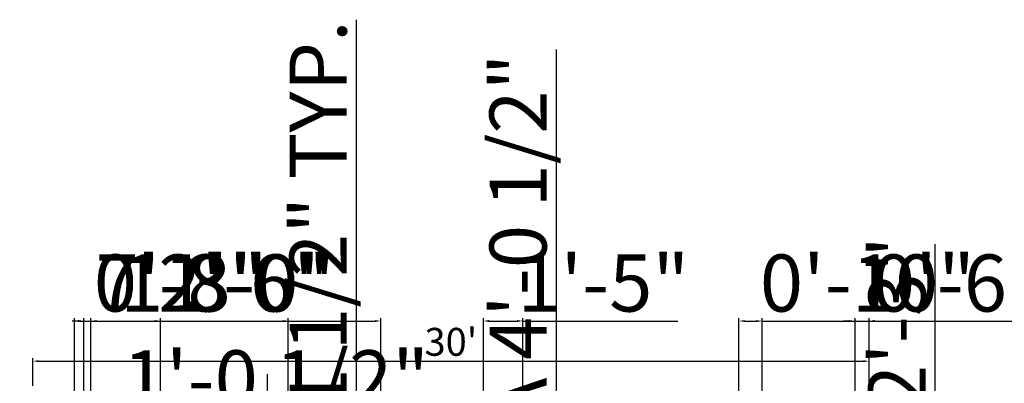
# Model space of a CAD drawing. Units: inches. Extents: x 1542 to 2523, y 1699 to 2449.
# Tile 6 of 7: x 1875 to 2299, y 2292 to 2449. Entities that reach past the tile are written whole.
import ezdxf

# ---------------------------------------------------------------- set-up
doc = ezdxf.new("R2010")
doc.units = ezdxf.units.IN
doc.layers.add('A-ANNO-DIMS', color=7, linetype='Continuous', lineweight=18)
doc.styles.get("Standard").update_dxf_attribs({"font": 'arial.ttf'})
doc.dimstyles.new('ISO-25', dxfattribs={"dimtxt": 24.5625, "dimasz": 2.5, "dimexe": 1.25, "dimexo": 0.625, "dimtad": 1, "dimlunit": 4, "dimtxsty": 'Standard', "dimcen": 2.5, "dimadec": 0, "dimazin": 0, "dimtfac": 10, "dimtmove": 0, "dimatfit": 3, "dimfxl": 1, "dimarcsym": 0})

# ---------------------------------------------------------------- blocks, each defined once
blk = doc.blocks.new('*D9')
at = {"layer": 'A-ANNO-DIMS', "color": 0, "lineweight": -2, "transparency": 16777216}
for p, q in [((1880.38, 2291.06), (1880.38, 2302.87)), ((2240.38, 2291.06), (2240.38, 2302.87)), ((1882.88, 2301.62), (2237.88, 2301.62))]:
    blk.add_line(p, q, dxfattribs=at)
at = {"layer": 'A-ANNO-DIMS', "color": 0, "transparency": 16777216}
for points in [[(1882.88, 2302.04), (1882.88, 2301.2), (1880.38, 2301.62)], [(2237.88, 2302.04), (2237.88, 2301.2), (2240.38, 2301.62)]]:
    blk.add_solid(points, dxfattribs=at)
at = {"layer": 'Defpoints', "color": 0, "transparency": 16777216}
for p in [(2240.38, 2301.62), (1880.38, 2290.44), (2240.38, 2290.44)]:
    blk.add_point(p, dxfattribs=at)
at = {"layer": 'A-ANNO-DIMS', "color": 0, "transparency": 16777216, "insert": (2060.38, 2308.37), "char_height": 12, "attachment_point": 5}
blk.add_mtext("30'", dxfattribs=at)
blk = doc.blocks.new('*D33')
at = {"layer": 'A-ANNO-DIMS', "color": 0, "lineweight": -2, "transparency": 16777216}
for p, q in [((1909.3, 2275.17), (1909.3, 2278.75)), ((1911.8, 2277.5), (1919.33, 2277.5)), ((1921.83, 2275.17), (1921.83, 2278.75)), ((1921.83, 2277.5), (2045.8, 2277.5))]:
    blk.add_line(p, q, dxfattribs=at)
at = {"layer": 'A-ANNO-DIMS', "color": 0, "transparency": 16777216}
for points in [[(1911.8, 2277.92), (1911.8, 2277.09), (1909.3, 2277.5)], [(1919.33, 2277.92), (1919.33, 2277.09), (1921.83, 2277.5)]]:
    blk.add_solid(points, dxfattribs=at)
at = {"layer": 'Defpoints', "color": 0, "transparency": 16777216}
for p in [(1921.83, 2277.5), (1909.3, 2274.54), (1921.83, 2274.54)]:
    blk.add_point(p, dxfattribs=at)
at = {"layer": 'A-ANNO-DIMS', "color": 0, "transparency": 16777216, "insert": (1985.06, 2290.83), "char_height": 24.562, "attachment_point": 5}
blk.add_mtext('1\'-0 1/2"', dxfattribs=at)
blk = doc.blocks.new('*D34')
at = {"layer": 'A-ANNO-DIMS', "color": 0, "lineweight": -2, "transparency": 16777216}
for p, q in [((1981.43, 2074.83), (1981.43, 2296.01)), ((1977.09, 2074.83), (1982.68, 2074.83)), ((1981.43, 2044.29), (1981.43, 2072.33)), ((1977.09, 2041.79), (1982.68, 2041.79))]:
    blk.add_line(p, q, dxfattribs=at)
at = {"layer": 'A-ANNO-DIMS', "color": 0, "transparency": 16777216}
for points in [[(1981.01, 2072.33), (1981.84, 2072.33), (1981.43, 2074.83)], [(1981.01, 2044.29), (1981.84, 2044.29), (1981.43, 2041.79)]]:
    blk.add_solid(points, dxfattribs=at)
at = {"layer": 'Defpoints', "color": 0, "transparency": 16777216}
for p in [(1976.47, 2074.83), (1981.43, 2074.83), (1976.47, 2041.79)]:
    blk.add_point(p, dxfattribs=at)
at = {"layer": 'A-ANNO-DIMS', "color": 0, "transparency": 16777216, "insert": (1968.1, 2186.67), "char_height": 24.5625, "attachment_point": 5, "rotation": 90}
blk.add_mtext('WC 2\'-9" TYP.', dxfattribs=at)
blk = doc.blocks.new('*D38')
at = {"layer": 'A-ANNO-DIMS', "color": 0, "lineweight": -2, "transparency": 16777216}
for p, q in [((1907.17, 2252.37), (1542.11, 2252.37)), ((1907.17, 2238.32), (1907.17, 2253.62)), ((2002.53, 2252.37), (1909.67, 2252.37)), ((2005.03, 2238.32), (2005.03, 2253.62))]:
    blk.add_line(p, q, dxfattribs=at)
at = {"layer": 'A-ANNO-DIMS', "color": 0, "transparency": 16777216}
for points in [[(1909.67, 2252.79), (1909.67, 2251.95), (1907.17, 2252.37)], [(2002.53, 2252.79), (2002.53, 2251.95), (2005.03, 2252.37)]]:
    blk.add_solid(points, dxfattribs=at)
at = {"layer": 'Defpoints', "color": 0, "transparency": 16777216}
for p in [(1907.17, 2252.37), (1907.17, 2237.69), (2005.03, 2237.69)]:
    blk.add_point(p, dxfattribs=at)
at = {"layer": 'A-ANNO-DIMS', "color": 0, "transparency": 16777216, "insert": (1723.39, 2266.45), "char_height": 24.5625, "attachment_point": 5}
blk.add_mtext('QUEEN BED 8\'-2" TYP.', dxfattribs=at)
blk = doc.blocks.new('*D39')
at = {"layer": 'A-ANNO-DIMS', "color": 0, "lineweight": -2, "transparency": 16777216}
for p, q in [((2019.71, 2237.69), (2019.71, 2448.53)), ((2005.65, 2237.69), (2020.96, 2237.69)), ((2019.71, 2166.8), (2019.71, 2235.19)), ((2005.65, 2164.3), (2020.96, 2164.3))]:
    blk.add_line(p, q, dxfattribs=at)
at = {"layer": 'A-ANNO-DIMS', "color": 0, "transparency": 16777216}
for points in [[(2019.29, 2235.19), (2020.12, 2235.19), (2019.71, 2237.69)], [(2019.29, 2166.8), (2020.12, 2166.8), (2019.71, 2164.3)]]:
    blk.add_solid(points, dxfattribs=at)
at = {"layer": 'Defpoints', "color": 0, "transparency": 16777216}
for p in [(2005.03, 2237.69), (2019.71, 2237.69), (2005.03, 2164.3)]:
    blk.add_point(p, dxfattribs=at)
at = {"layer": 'A-ANNO-DIMS', "color": 0, "transparency": 16777216, "insert": (2006.38, 2344.36), "char_height": 24.5625, "attachment_point": 5, "rotation": 90}
blk.add_mtext('6\'-1 1/2" TYP.', dxfattribs=at)
blk = doc.blocks.new('*D44')
at = {"layer": 'A-ANNO-DIMS', "color": 0, "lineweight": -2, "transparency": 16777216}
for p, q in [((2105.8, 2206.61), (2105.8, 2435.72)), ((2099.19, 2206.61), (2107.05, 2206.61)), ((2105.8, 2160.85), (2105.8, 2204.11)), ((2099.19, 2158.35), (2107.05, 2158.35))]:
    blk.add_line(p, q, dxfattribs=at)
at = {"layer": 'A-ANNO-DIMS', "color": 0, "transparency": 16777216}
for points in [[(2105.39, 2204.11), (2106.22, 2204.11), (2105.8, 2206.61)], [(2105.39, 2160.85), (2106.22, 2160.85), (2105.8, 2158.35)]]:
    blk.add_solid(points, dxfattribs=at)
at = {"layer": 'Defpoints', "color": 0, "transparency": 16777216}
for p in [(2098.56, 2206.61), (2105.8, 2206.61), (2098.56, 2158.35)]:
    blk.add_point(p, dxfattribs=at)
at = {"layer": 'A-ANNO-DIMS', "color": 0, "transparency": 16777216, "insert": (2092.47, 2322.42), "char_height": 24.5625, "attachment_point": 5, "rotation": 90}
blk.add_mtext('SOFA 4\'-0 1/2"', dxfattribs=at)
blk = doc.blocks.new('*D48')
at = {"layer": 'A-ANNO-DIMS', "color": 0, "lineweight": -2, "transparency": 16777216}
for p, q in [((1905.38, 2077.06), (1905.38, 2320.14)), ((1907.88, 2318.89), (1932.88, 2318.89)), ((1935.38, 2077.06), (1935.38, 2320.14)), ((1935.38, 2318.89), (2004.84, 2318.89))]:
    blk.add_line(p, q, dxfattribs=at)
at = {"layer": 'A-ANNO-DIMS', "color": 0, "transparency": 16777216}
for points in [[(1907.88, 2319.31), (1907.88, 2318.47), (1905.38, 2318.89)], [(1932.88, 2319.31), (1932.88, 2318.47), (1935.38, 2318.89)]]:
    blk.add_solid(points, dxfattribs=at)
at = {"layer": 'Defpoints', "color": 0, "transparency": 16777216}
for p in [(1935.38, 2318.89), (1905.38, 2076.44), (1935.38, 2076.44)]:
    blk.add_point(p, dxfattribs=at)
at = {"layer": 'A-ANNO-DIMS', "color": 0, "transparency": 16777216, "insert": (1971.36, 2332.05), "char_height": 24.562, "attachment_point": 5}
blk.add_mtext('2\'-6"', dxfattribs=at)
blk = doc.blocks.new('*D50')
at = {"layer": 'A-ANNO-DIMS', "color": 0, "lineweight": -2, "transparency": 16777216}
for p, q in [((2268.83, 2282.44), (2268.83, 2351.9)), ((1987.01, 2282.44), (2270.08, 2282.44)), ((2268.83, 2257.94), (2268.83, 2279.94)), ((1987.01, 2255.44), (2270.08, 2255.44))]:
    blk.add_line(p, q, dxfattribs=at)
at = {"layer": 'A-ANNO-DIMS', "color": 0, "transparency": 16777216}
for points in [[(2268.42, 2279.94), (2269.25, 2279.94), (2268.83, 2282.44)], [(2268.42, 2257.94), (2269.25, 2257.94), (2268.83, 2255.44)]]:
    blk.add_solid(points, dxfattribs=at)
at = {"layer": 'Defpoints', "color": 0, "transparency": 16777216}
for p in [(1986.38, 2282.44), (2268.83, 2282.44), (1986.38, 2255.44)]:
    blk.add_point(p, dxfattribs=at)
at = {"layer": 'A-ANNO-DIMS', "color": 0, "transparency": 16777216, "insert": (2255.66, 2318.42), "char_height": 24.562, "attachment_point": 5, "rotation": 90}
blk.add_mtext('2\'-3"', dxfattribs=at)
blk = doc.blocks.new('*D54')
at = {"layer": 'A-ANNO-DIMS', "color": 0, "lineweight": -2, "transparency": 16777216}
for p, q in [((2231.88, 2318.89), (2229.38, 2318.89)), ((2234.38, 2285.06), (2234.38, 2320.14)), ((2234.38, 2318.89), (2240.38, 2318.89)), ((2240.38, 2291.06), (2240.38, 2320.14)), ((2242.88, 2318.89), (2311.93, 2318.89))]:
    blk.add_line(p, q, dxfattribs=at)
at = {"layer": 'A-ANNO-DIMS', "color": 0, "transparency": 16777216}
for points in [[(2231.88, 2319.31), (2231.88, 2318.47), (2234.38, 2318.89)], [(2242.88, 2319.31), (2242.88, 2318.47), (2240.38, 2318.89)]]:
    blk.add_solid(points, dxfattribs=at)
at = {"layer": 'Defpoints', "color": 0, "transparency": 16777216}
for p in [(2240.38, 2318.89), (2240.38, 2290.44), (2234.38, 2284.44)]:
    blk.add_point(p, dxfattribs=at)
at = {"layer": 'A-ANNO-DIMS', "color": 0, "transparency": 16777216, "insert": (2278.65, 2332.05), "char_height": 24.562, "attachment_point": 5}
blk.add_mtext('0\'-6"', dxfattribs=at)
blk = doc.blocks.new('*D61')
at = {"layer": 'A-ANNO-DIMS', "color": 0, "lineweight": -2, "transparency": 16777216}
for p, q in [((1898.38, 2253.06), (1898.38, 2320.14)), ((1900.88, 2318.89), (2027.64, 2318.89)), ((2030.14, 2253.06), (2030.14, 2320.14))]:
    blk.add_line(p, q, dxfattribs=at)
at = {"layer": 'A-ANNO-DIMS', "color": 0, "transparency": 16777216}
for points in [[(1900.88, 2319.31), (1900.88, 2318.47), (1898.38, 2318.89)], [(2027.64, 2319.31), (2027.64, 2318.47), (2030.14, 2318.89)]]:
    blk.add_solid(points, dxfattribs=at)
at = {"layer": 'Defpoints', "color": 0, "transparency": 16777216}
for p in [(2030.14, 2318.89), (1898.38, 2252.44), (2030.14, 2252.44)]:
    blk.add_point(p, dxfattribs=at)
at = {"layer": 'A-ANNO-DIMS', "color": 0, "transparency": 16777216, "insert": (1964.26, 2332.05), "char_height": 24.562, "attachment_point": 5}
blk.add_mtext('11\'-0"', dxfattribs=at)
blk = doc.blocks.new('*D62')
at = {"layer": 'A-ANNO-DIMS', "color": 0, "lineweight": -2, "transparency": 16777216}
for p, q in [((2074.38, 2249.06), (2074.38, 2320.14)), ((2076.88, 2318.89), (2088.88, 2318.89)), ((2091.38, 2249.06), (2091.38, 2320.14)), ((2091.38, 2318.89), (2158.11, 2318.89))]:
    blk.add_line(p, q, dxfattribs=at)
at = {"layer": 'A-ANNO-DIMS', "color": 0, "transparency": 16777216}
for points in [[(2076.88, 2319.31), (2076.88, 2318.47), (2074.38, 2318.89)], [(2088.88, 2319.31), (2088.88, 2318.47), (2091.38, 2318.89)]]:
    blk.add_solid(points, dxfattribs=at)
at = {"layer": 'Defpoints', "color": 0, "transparency": 16777216}
for p in [(2091.38, 2318.89), (2074.38, 2248.44), (2091.38, 2248.44)]:
    blk.add_point(p, dxfattribs=at)
at = {"layer": 'A-ANNO-DIMS', "color": 0, "transparency": 16777216, "insert": (2126, 2332.05), "char_height": 24.562, "attachment_point": 5}
blk.add_mtext('1\'-5"', dxfattribs=at)
blk = doc.blocks.new('*D63')
at = {"layer": 'A-ANNO-DIMS', "color": 0, "lineweight": -2, "transparency": 16777216}
for p, q in [((2184.39, 2249.06), (2184.39, 2320.14)), ((2186.89, 2318.89), (2191.88, 2318.89)), ((2194.38, 2249.06), (2194.38, 2320.14)), ((2194.38, 2318.89), (2282.51, 2318.89))]:
    blk.add_line(p, q, dxfattribs=at)
at = {"layer": 'A-ANNO-DIMS', "color": 0, "transparency": 16777216}
for points in [[(2186.89, 2319.31), (2186.89, 2318.47), (2184.39, 2318.89)], [(2191.88, 2319.31), (2191.88, 2318.47), (2194.38, 2318.89)]]:
    blk.add_solid(points, dxfattribs=at)
at = {"layer": 'Defpoints', "color": 0, "transparency": 16777216}
for p in [(2194.38, 2318.89), (2184.39, 2248.44), (2194.38, 2248.44)]:
    blk.add_point(p, dxfattribs=at)
at = {"layer": 'A-ANNO-DIMS', "color": 0, "transparency": 16777216, "insert": (2239.7, 2332.05), "char_height": 24.562, "attachment_point": 5}
blk.add_mtext('0\'-10"', dxfattribs=at)
blk = doc.blocks.new('*D65')
at = {"layer": 'A-ANNO-DIMS', "color": 0, "lineweight": -2, "transparency": 16777216}
for p, q in [((1898.38, 2285.06), (1898.38, 2320.14)), ((1900.88, 2318.89), (1987.88, 2318.89)), ((1990.38, 2285.06), (1990.38, 2320.14))]:
    blk.add_line(p, q, dxfattribs=at)
at = {"layer": 'A-ANNO-DIMS', "color": 0, "transparency": 16777216}
for points in [[(1900.88, 2319.31), (1900.88, 2318.47), (1898.38, 2318.89)], [(1987.88, 2319.31), (1987.88, 2318.47), (1990.38, 2318.89)]]:
    blk.add_solid(points, dxfattribs=at)
at = {"layer": 'Defpoints', "color": 0, "transparency": 16777216}
for p in [(1990.38, 2318.89), (1898.38, 2284.44), (1990.38, 2284.44)]:
    blk.add_point(p, dxfattribs=at)
at = {"layer": 'A-ANNO-DIMS', "color": 0, "transparency": 16777216, "insert": (1944.38, 2332.05), "char_height": 24.562, "attachment_point": 5}
blk.add_mtext('7\'-8"', dxfattribs=at)
blk = doc.blocks.new('*D66')
at = {"layer": 'A-ANNO-DIMS', "color": 0, "lineweight": -2, "transparency": 16777216}
for p, q in [((1851.93, 2286.94), (1851.93, 2413.22)), ((1901.76, 2284.44), (1850.68, 2284.44)), ((1851.93, 2279.86), (1851.93, 2284.44)), ((1901.76, 2279.86), (1850.68, 2279.86)), ((1851.93, 2277.36), (1851.93, 2274.86))]:
    blk.add_line(p, q, dxfattribs=at)
at = {"layer": 'A-ANNO-DIMS', "color": 0, "transparency": 16777216}
for points in [[(1851.52, 2286.94), (1852.35, 2286.94), (1851.93, 2284.44)], [(1851.52, 2277.36), (1852.35, 2277.36), (1851.93, 2279.86)]]:
    blk.add_solid(points, dxfattribs=at)
at = {"layer": 'Defpoints', "color": 0, "transparency": 16777216}
for p in [(1851.93, 2284.44), (1902.38, 2284.44), (1902.38, 2279.86)]:
    blk.add_point(p, dxfattribs=at)
at = {"layer": 'A-ANNO-DIMS', "color": 0, "transparency": 16777216, "insert": (1838.61, 2351.33), "char_height": 24.562, "attachment_point": 5, "rotation": 90}
blk.add_mtext('0\'-4 1/2"', dxfattribs=at)
blk = doc.blocks.new('*D69')
at = {"layer": 'A-ANNO-DIMS', "color": 0, "lineweight": -2, "transparency": 16777216}
for p, q in [((1899.88, 2318.89), (1897.38, 2318.89)), ((1902.38, 2077.06), (1902.38, 2320.14)), ((1902.38, 2318.89), (1905.38, 2318.89)), ((1905.38, 2077.06), (1905.38, 2320.14)), ((1907.88, 2318.89), (1976.93, 2318.89))]:
    blk.add_line(p, q, dxfattribs=at)
at = {"layer": 'A-ANNO-DIMS', "color": 0, "transparency": 16777216}
for points in [[(1899.88, 2319.31), (1899.88, 2318.47), (1902.38, 2318.89)], [(1907.88, 2319.31), (1907.88, 2318.47), (1905.38, 2318.89)]]:
    blk.add_solid(points, dxfattribs=at)
at = {"layer": 'Defpoints', "color": 0, "transparency": 16777216}
for p in [(1905.38, 2318.89), (1902.38, 2076.44), (1905.38, 2076.44)]:
    blk.add_point(p, dxfattribs=at)
at = {"layer": 'A-ANNO-DIMS', "color": 0, "transparency": 16777216, "insert": (1943.65, 2332.06), "char_height": 24.562, "attachment_point": 5}
blk.add_mtext('0\'-3"', dxfattribs=at)

msp = doc.modelspace()

# ---------------------------------------------------------------- dimensions: what is measured, and where the dimension line sits
at = {"layer": 'A-ANNO-DIMS'}
for base, p1, p2, angle, text, picture, middle in [((2019.707, 2237.692), (2005.029, 2164.301), (2005.029, 2237.692), 90, '<> TYP.', '*D39', (2006.382, 2344.362)), ((2105.802, 2206.606), (2098.565, 2158.354), (2098.565, 2206.606), 90, 'SOFA <>', '*D44', (2092.469, 2322.416)), ((1907.173, 2252.371), (2005.029, 2237.692), (1907.173, 2237.692), 180, 'QUEEN BED <> TYP.', '*D38', (1723.39, 2266.45)), ((1981.426, 2074.834), (1976.469, 2041.788), (1976.469, 2074.834), 90, 'WC <> TYP.', '*D34', (1968.101, 2186.673))]:
    dim = msp.add_linear_dim(base=base, p1=p1, p2=p2, angle=angle, text=text, dimstyle='ISO-25', override={"dimdec": 1, "dimlfac": 1, "dimrnd": 0, "dimzin": 1, "dimdsep": 46, "dimlunit": 4, "dimfrac": 2}, dxfattribs=at)
    dim.commit()
    dim.dimension.update_dxf_attribs({"geometry": picture, "text_midpoint": middle})
for base, p1, p2, picture, middle in [((1851.933, 2284.439), (1902.383, 2279.859), (1902.383, 2284.439), '*D66', (1838.607, 2351.328)), ((2268.833, 2282.439), (1986.383, 2255.439), (1986.383, 2282.439), '*D50', (2255.658, 2318.42))]:
    dim = msp.add_linear_dim(base=base, p1=p1, p2=p2, angle=90, dimstyle='ISO-25', override={"dimdec": 1, "dimlfac": 1, "dimrnd": 0, "dimzin": 1, "dimdsep": 46, "dimlunit": 4, "dimfrac": 2}, dxfattribs=at)
    dim.commit()
    dim.dimension.update_dxf_attribs({"geometry": picture, "text_midpoint": middle})
for base, p1, p2, override, picture, middle in [((1905.383, 2318.889), (1902.383, 2076.439), (1905.383, 2076.439), {"dimdec": 1, "dimlfac": 1, "dimrnd": 0, "dimzin": 1, "dimdsep": 46, "dimlunit": 4, "dimfrac": 2}, '*D69', (1943.654, 2332.063)), ((2030.138, 2318.889), (1898.383, 2252.439), (2030.138, 2252.439), {"dimdec": 1, "dimlfac": 1, "dimrnd": 0, "dimzin": 1, "dimdsep": 46, "dimlunit": 4, "dimfrac": 2}, '*D61', (1964.26, 2332.055)), ((1990.383, 2318.889), (1898.383, 2284.439), (1990.383, 2284.439), {"dimdec": 1, "dimlfac": 1, "dimrnd": 0, "dimzin": 1, "dimdsep": 46, "dimlunit": 4, "dimfrac": 2}, '*D65', (1944.383, 2332.055)), ((1935.383, 2318.889), (1905.383, 2076.439), (1935.383, 2076.439), {"dimdec": 1, "dimlfac": 1, "dimrnd": 0, "dimzin": 1, "dimdsep": 46, "dimlunit": 4, "dimfrac": 2}, '*D48', (1971.364, 2332.055)), ((2091.383, 2318.889), (2074.383, 2248.439), (2091.383, 2248.439), {"dimdec": 1, "dimlfac": 1, "dimrnd": 0, "dimzin": 1, "dimdsep": 46, "dimlunit": 4, "dimfrac": 2}, '*D62', (2125.998, 2332.055)), ((2194.383, 2318.889), (2184.395, 2248.439), (2194.383, 2248.439), {"dimdec": 1, "dimlfac": 1, "dimrnd": 0, "dimzin": 1, "dimdsep": 46, "dimlunit": 4, "dimfrac": 2}, '*D63', (2239.696, 2332.055)), ((2240.383, 2318.889), (2234.383, 2284.439), (2240.383, 2290.439), {"dimdec": 1, "dimlfac": 1, "dimrnd": 0, "dimzin": 1, "dimdsep": 46, "dimlunit": 4, "dimfrac": 2}, '*D54', (2278.654, 2332.055)), ((1921.831, 2277.503), (1909.3, 2274.545), (1921.831, 2274.545), {"dimdec": 1, "dimlfac": 1, "dimrnd": 0, "dimzin": 1, "dimdsep": 46, "dimlunit": 4, "dimfrac": 2}, '*D33', (1985.063, 2290.828)), ((2240.383, 2301.619), (1880.383, 2290.439), (2240.383, 2290.439), {"dimtxt": 12, "dimclrd": 0, "dimclre": 0, "dimclrt": 0}, '*D9', (2060.383, 2308.375))]:
    dim = msp.add_linear_dim(base=base, p1=p1, p2=p2, dimstyle='ISO-25', override=override, dxfattribs=at)
    dim.commit()
    dim.dimension.update_dxf_attribs({"geometry": picture, "text_midpoint": middle})

doc.saveas('drawing.dxf')
